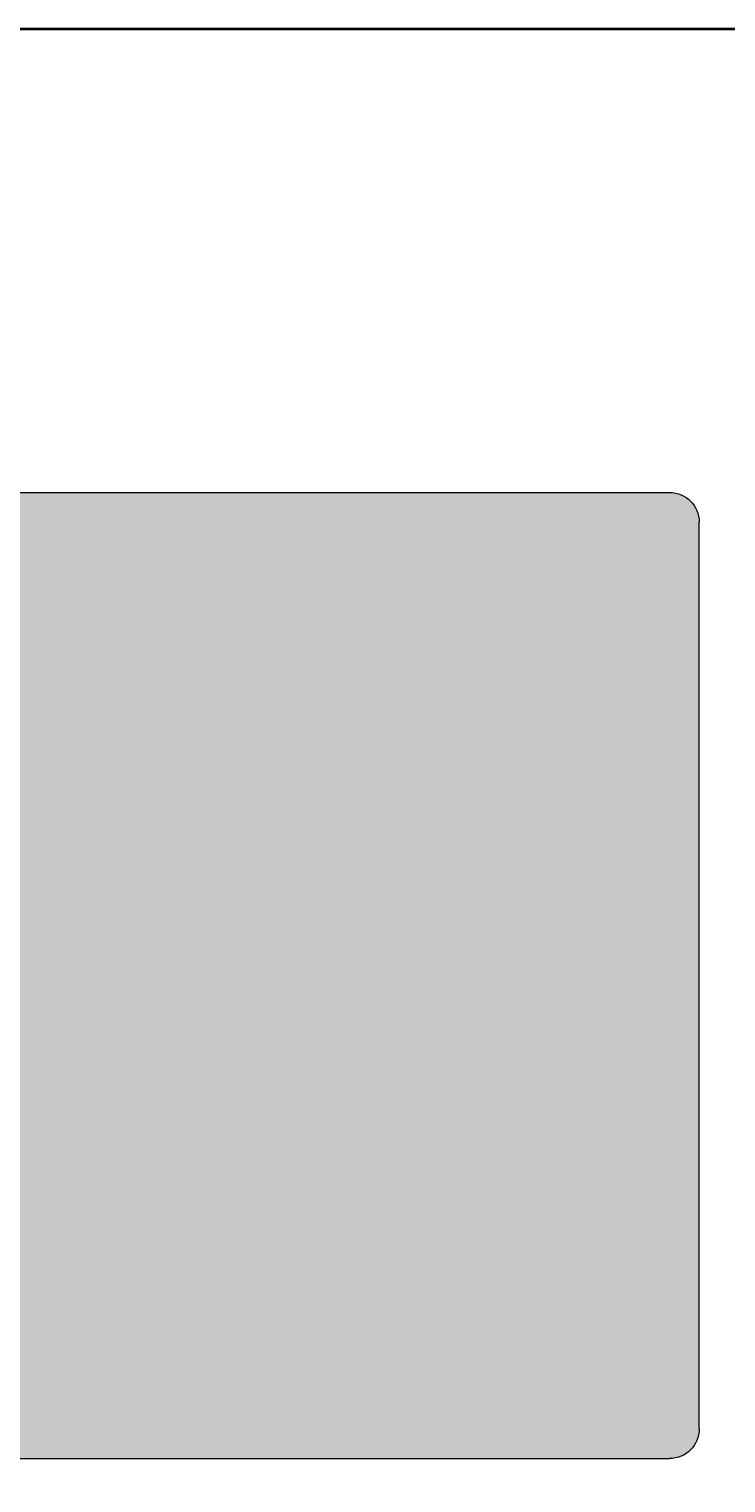
# Model space of a CAD drawing. Units: millimetres. Extents: x 27017497 to 27018854, y 7058029 to 7059154.
# Tile 86 of 91: x 27018362 to 27018399, y 7058503 to 7058581. Entities that reach past the tile are written whole.
import ezdxf

# ---------------------------------------------------------------- set-up
doc = ezdxf.new("R2010")
doc.units = ezdxf.units.MM
for name, color, linetype, lineweight in [('A-ANNO-DIMS', 2, 'Continuous', 18), ('A-FURN', 8, 'Continuous', 18), ('A-WALL', 7, 'Continuous', 35)]:
    doc.layers.add(name, color=color, linetype=linetype, lineweight=lineweight)
doc.layers.add('A-FURN-PATT', color=177, linetype='Continuous', lineweight=13, true_color=0x293189)
doc.styles.get("Standard").update_dxf_attribs({"font": 'arial.ttf'})
doc.dimstyles.get("Standard").update_dxf_attribs({"dimtxt": 0.18, "dimasz": 0.18, "dimexe": 0.18, "dimexo": 0.0625, "dimgap": 0.09, "dimtad": 0, "dimtih": 1, "dimtoh": 1, "dimdec": 4, "dimzin": 0, "dimdsep": 46, "dimtxsty": 'Standard', "dimcen": 0.09, "dimadec": 0, "dimazin": 0, "dimtfac": 1, "dimtdec": 4, "dimtofl": 0, "dimtmove": 0, "dimatfit": 3, "dimfxl": 1, "dimtolj": 1, "dimtzin": 0, "dimarcsym": 0})

# ---------------------------------------------------------------- blocks, each defined once
blk = doc.blocks.new('CAMMAT')
for p, q in [((-0.65, -0.8139), (-0.65, -1.93)), ((0.65, -0.8204), (0.65, -1.93)), ((0.61, -1.97), (-0.61, -1.97))]:
    blk.add_line(p, q)
for centre, start, end in [((-0.61, -1.93), 180, 270), ((0.61, -1.93), 270, 360)]:
    blk.add_arc(centre, 0.04, start, end)
blk = doc.blocks.new('*D48')
at = {"layer": 'A-ANNO-DIMS', "color": 0, "lineweight": -2, "transparency": 16777216}
for p, q in [((27018463.498, 7058622.912), (27017497.536, 7058622.912)), ((27017497.716, 7058622.732), (27017497.716, 7058357.753)), ((27017497.716, 7058092.41), (27017497.716, 7058357.389)), ((27018555.129, 7058092.23), (27017497.536, 7058092.23))]:
    blk.add_line(p, q, dxfattribs=at)
at = {"layer": 'A-ANNO-DIMS', "color": 0, "transparency": 16777216}
for points in [[(27017497.686, 7058622.732), (27017497.746, 7058622.732), (27017497.716, 7058622.912)], [(27017497.686, 7058092.41), (27017497.746, 7058092.41), (27017497.716, 7058092.23)]]:
    blk.add_solid(points, dxfattribs=at)
at = {"layer": 'Defpoints', "color": 0, "transparency": 16777216}
for p in [(27018463.561, 7058622.912), (27017497.716, 7058092.23), (27018555.192, 7058092.23)]:
    blk.add_point(p, dxfattribs=at)
at = {"layer": 'A-ANNO-DIMS', "color": 0, "transparency": 16777216, "insert": (27017497.716, 7058357.571), "char_height": 0.18, "attachment_point": 5}
blk.add_mtext('\\A1;530.7', dxfattribs=at)
blk = doc.blocks.new('*D50')
at = {"layer": 'A-ANNO-DIMS', "color": 0, "lineweight": -2, "transparency": 16777216}
for p, q in [((27018223.668, 7058580.912), (27018854.236, 7058580.912)), ((27018854.056, 7058580.732), (27018854.056, 7058511.344)), ((27018854.056, 7058441.592), (27018854.056, 7058510.98)), ((27018223.668, 7058441.412), (27018854.236, 7058441.412))]:
    blk.add_line(p, q, dxfattribs=at)
at = {"layer": 'A-ANNO-DIMS', "color": 0, "transparency": 16777216}
for points in [[(27018854.026, 7058580.732), (27018854.086, 7058580.732), (27018854.056, 7058580.912)], [(27018854.026, 7058441.592), (27018854.086, 7058441.592), (27018854.056, 7058441.412)]]:
    blk.add_solid(points, dxfattribs=at)
at = {"layer": 'Defpoints', "color": 0, "transparency": 16777216}
for p in [(27018223.606, 7058580.912), (27018223.606, 7058441.412), (27018854.056, 7058441.412)]:
    blk.add_point(p, dxfattribs=at)
at = {"layer": 'A-ANNO-DIMS', "color": 0, "transparency": 16777216, "insert": (27018854.056, 7058511.162), "char_height": 0.18, "attachment_point": 5}
blk.add_mtext('\\A1;139.5', dxfattribs=at)

msp = doc.modelspace()

# ---------------------------------------------------------------- hatches: boundary and pattern name
at = {"layer": 'A-FURN-PATT'}
h = msp.add_hatch(color=256, dxfattribs=at)
h.dxf.hatch_style = 1
h.paths.add_polyline_path([(27018398.067, 7058554.497, 0.414214), (27018396.474, 7058556.09), (27018352.018, 7058556.09), (27018352.202, 7058552.834), (27018352.581, 7058547.929), (27018353.082, 7058544.346), (27018353.818, 7058541.828), (27018354.899, 7058540.115), (27018356.437, 7058538.948), (27018358.543, 7058538.068), (27018361.329, 7058537.215), (27018358.524, 7058536.613), (27018356.284, 7058536.07), (27018354.381, 7058535.48), (27018352.588, 7058534.736), (27018350.68, 7058533.729), (27018348.431, 7058532.354), (27018345.612, 7058530.503), (27018341.998, 7058528.068), (27018345.612, 7058525.633), (27018348.431, 7058523.782), (27018350.68, 7058522.407), (27018352.588, 7058521.4), (27018354.381, 7058520.656), (27018356.284, 7058520.066), (27018358.524, 7058519.523), (27018361.329, 7058518.92), (27018358.543, 7058518.068), (27018356.437, 7058517.188), (27018354.899, 7058516.021), (27018353.818, 7058514.308), (27018353.082, 7058511.79), (27018352.581, 7058508.207), (27018352.28, 7058504.311), (27018396.474, 7058504.311, 0.414214), (27018398.067, 7058505.904)])
h.paths.add_polyline_path([(27018356.437, 7058538.948), (27018354.899, 7058540.115), (27018353.818, 7058541.828), (27018353.082, 7058544.346), (27018352.581, 7058547.929), (27018352.202, 7058552.834), (27018351.835, 7058559.322), (27018341.998, 7058528.068), (27018345.612, 7058530.503), (27018348.431, 7058532.354), (27018350.68, 7058533.729), (27018352.588, 7058534.736), (27018354.381, 7058535.48), (27018356.284, 7058536.07), (27018358.524, 7058536.613), (27018361.329, 7058537.215), (27018358.543, 7058538.068)])
h.paths.add_polyline_path([(27018358.543, 7058518.068), (27018361.329, 7058518.92), (27018358.524, 7058519.523), (27018356.284, 7058520.066), (27018354.381, 7058520.656), (27018352.588, 7058521.4), (27018350.68, 7058522.407), (27018348.431, 7058523.782), (27018345.612, 7058525.633), (27018341.998, 7058528.068), (27018351.835, 7058496.813), (27018352.202, 7058503.301), (27018352.581, 7058508.207), (27018353.082, 7058511.79), (27018353.818, 7058514.308), (27018354.899, 7058516.021), (27018356.437, 7058517.188)])
h.paths.add_polyline_path([(27018351.324, 7058557.699), (27018340.191, 7058557.699), (27018340.191, 7058503.014), (27018349.884, 7058503.014), (27018341.998, 7058528.068)])
h.paths.add_polyline_path([(27018340.191, 7058556.09), (27018323.983, 7058556.09, 0.414214), (27018322.39, 7058554.497), (27018322.39, 7058505.904, 0.414214), (27018323.983, 7058504.311), (27018340.191, 7058504.311)])
h.paths.add_polyline_path([(27018337.107, 7058532.051, -0.414214), (27018335.912, 7058530.856), (27018326.353, 7058530.856, -0.414214), (27018325.158, 7058532.051), (27018325.158, 7058553.51, -0.414214), (27018326.353, 7058554.705), (27018335.912, 7058554.705, -0.414214), (27018337.107, 7058553.51)], flags=0)
h.paths.add_polyline_path([(27018337.107, 7058527.914), (27018337.107, 7058506.454, -0.414214), (27018335.912, 7058505.259), (27018326.353, 7058505.259, -0.414214), (27018325.158, 7058506.454), (27018325.158, 7058527.914, -0.414214), (27018326.353, 7058529.109), (27018335.912, 7058529.109, -0.414214)], flags=0)
h.paths.add_polyline_path([(27018338.322, 7058577.2), (27018322.39, 7058577.2), (27018322.39, 7058557.285), (27018338.322, 7058557.285)])
h.paths.add_polyline_path([(27018323.748, 7058567.284, -1), (27018335.697, 7058567.284, -1)], flags=16)
h.paths.add_polyline_path([(27018326.023, 7058567.284, -1), (27018333.423, 7058567.284, -1)], flags=0)
h.paths.add_polyline_path([(27018338.322, 7058503.116), (27018322.39, 7058503.116), (27018322.39, 7058483.201), (27018338.322, 7058483.201)])
h.paths.add_polyline_path([(27018335.697, 7058493.391, -1), (27018323.748, 7058493.391, -1)], flags=16)
h.paths.add_polyline_path([(27018333.423, 7058493.391, -1), (27018326.023, 7058493.391, -1)], flags=0)
h.paths.add_polyline_path([(27018337.107, 7058527.914, 0.414214), (27018335.912, 7058529.109), (27018326.353, 7058529.109, 0.414214), (27018325.158, 7058527.914), (27018325.158, 7058506.454, 0.414214), (27018326.353, 7058505.259), (27018335.912, 7058505.259, 0.414214), (27018337.107, 7058506.454)], flags=16)
h.paths.add_polyline_path([(27018337.107, 7058553.51, 0.414214), (27018335.912, 7058554.705), (27018326.353, 7058554.705, 0.414214), (27018325.158, 7058553.51), (27018325.158, 7058532.051, 0.414214), (27018326.353, 7058530.856), (27018335.912, 7058530.856, 0.414214), (27018337.107, 7058532.051)], flags=16)

# ---------------------------------------------------------------- linework, layer by layer
at = {"layer": 'A-WALL'}
msp.add_line((27018729.106, 7058580.912), (27018319.606, 7058580.912), dxfattribs=at)

# ---------------------------------------------------------------- block references
at = {"layer": 'A-FURN', "xscale": -39.82996475819422, "yscale": 39.82996475819422, "zscale": 39.82996475819422, "rotation": 90}
msp.add_blockref('CAMMAT', (27018319.602, 7058530.2), dxfattribs=at)

# ---------------------------------------------------------------- dimensions: what is measured, and where the dimension line sits
at = {"layer": 'A-ANNO-DIMS'}
for base, p1, p2, picture, middle in [((27017497.716, 7058092.23), (27018463.561, 7058622.912), (27018555.192, 7058092.23), '*D48', (27017497.716, 7058357.571)), ((27018854.056, 7058441.412), (27018223.606, 7058580.912), (27018223.606, 7058441.412), '*D50', (27018854.056, 7058511.162))]:
    dim = msp.add_linear_dim(base=base, p1=p1, p2=p2, angle=90, dimstyle='Standard', override={"dimdec": 1, "dimlfac": 1, "dimrnd": 0, "dimzin": 0, "dimdsep": 46, "dimlunit": 2}, dxfattribs=at)
    dim.commit()
    dim.dimension.update_dxf_attribs({"geometry": picture, "text_midpoint": middle})

doc.saveas('drawing.dxf')
